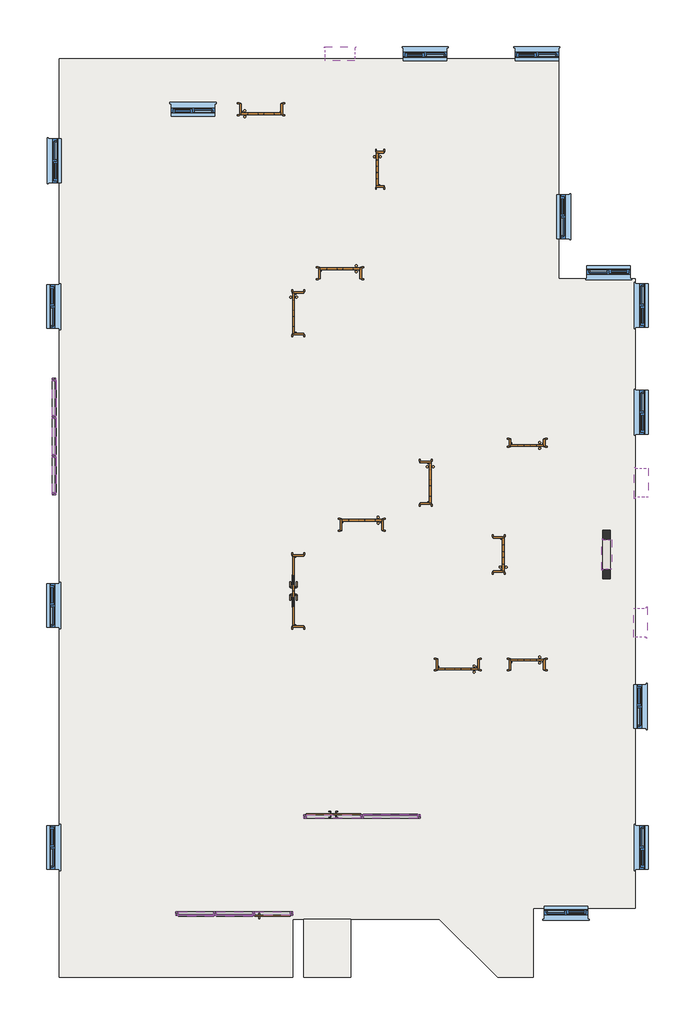
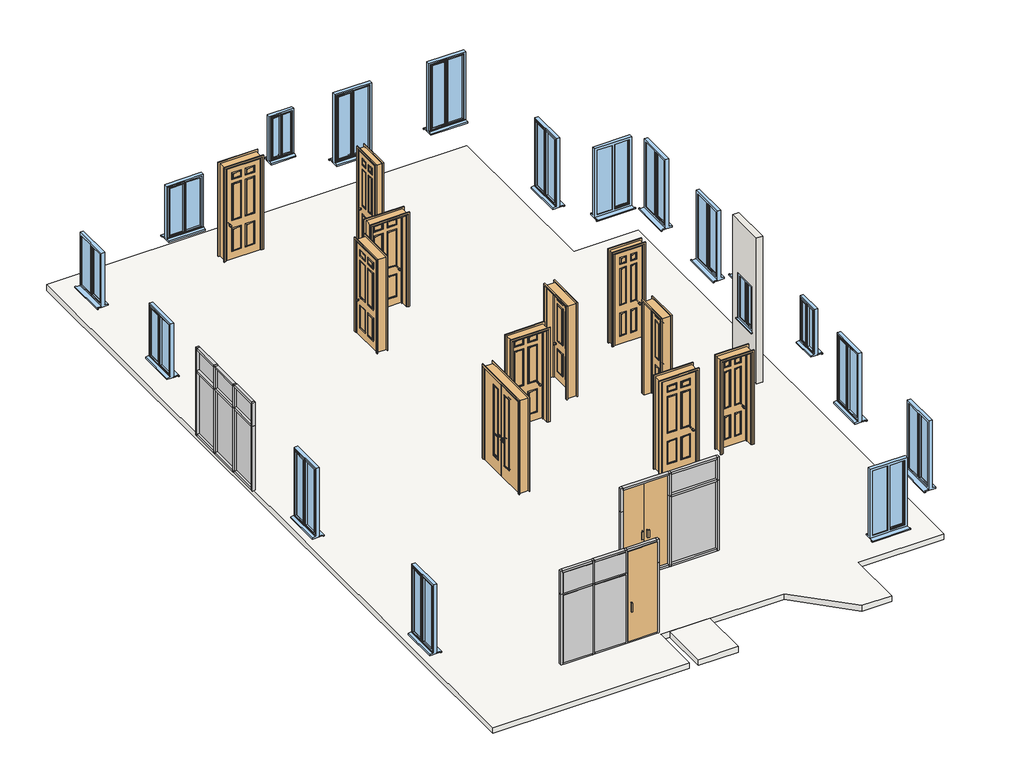
# One storey: 44 members, 18 windows, 13 doors, 12 plates, 2 slabs, 1 wall.
"""IFC4 building model written with IfcOpenShell, lengths in millimetres."""

from ifc_helpers import new_model, si_unit, frame, origin, place, context, project, spatial, polyline, outline, extrude, transform, mapped, element, save
from components import doors_intdbl_2_d4_7d0a9876, doors_intsgl_6_01_d1_adb953bf, doors_intsgl_6_01_d1_21fcec07, doors_intsgl_6_d2_0bf64c77, doors_intsgl_6_d2_b603f254, doors_intsgl_6_d2_ad12cddb, m_door_curtain_wall_double_glass_m_door_curtain_wall_double_ad7744c8, m_door_curtain_wall_single_glass_m_door_curtain_wall_single_7bb093da, rectangular_mullion_main_mullions_fa6a4a93, rectangular_mullion_main_mullions_32a4afb2, rectangular_mullion_main_mullions_07477f58, rectangular_mullion_main_mullions_65d9d1a0, rectangular_mullion_main_mullions_4e228a20, rectangular_mullion_main_mullions_6707c5fc, rectangular_mullion_main_mullions_bcbd968b, rectangular_mullion_main_mullions_6d09e4bf, rectangular_mullion_main_mullions_5bed117f, rectangular_mullion_main_mullions_97ba9194, rectangular_mullion_main_mullions_1ff2eda8, rectangular_mullion_main_mullions_8c683149, system_panel_glazed_41825f56, system_panel_glazed_b6ba8a14, system_panel_glazed_f19c5426, system_panel_glazed_62604723, system_panel_glazed_3b80f955, system_panel_glazed_1e8a61fc, system_panel_glazed_efe6ecb3, system_panel_glazed_1d3ea9f9, w1_9a3d44e1, w2_02e3e303, w2_3d16f0f7, w3_c0944c91

model = new_model("IFC4")

# Units and contexts
model_context = context("Model", 3, world=origin())
ifc_project = project(units=[si_unit("LENGTHUNIT", "METRE", prefix="MILLI")], contexts=[model_context])

# Site, building, storey
site = spatial("IfcSite", under=ifc_project)
building = spatial("IfcBuilding", under=site)
storey = spatial("IfcBuildingStorey", under=building, Elevation=600.0)

# Doors
placement = place(None, origin())
doors_intdbl_2_d4_shape = doors_intdbl_2_d4_7d0a9876(model_context)
element("IfcDoor", 1, ObjectType="Doors_IntDbl_2 : D4", at=placement, inside=storey, context=model_context, shape_type="MappedRepresentation", body=[
    mapped(doors_intdbl_2_d4_shape, transform((-3747.9564803, -5872.5265, 600.0), x_axis=(0.0, 1.0, 0.0), y_axis=(-1.0, 0.0, 0.0), z_axis=(0.0, 0.0, 1.0))),
])
doors_intsgl_6_01_d1_shape = doors_intsgl_6_01_d1_adb953bf(model_context)
element("IfcDoor", 2, ObjectType="Doors_IntSgl_6 : 01-D1", at=placement, inside=storey, context=model_context, shape_type="MappedRepresentation", body=[
    mapped(doors_intsgl_6_01_d1_shape, transform((-460.4564803, -7385.0265, 600.0), x_axis=(-1.0, 0.0, 0.0), y_axis=(0.0, -1.0, 0.0), z_axis=(0.0, 0.0, 1.0))),
])
element("IfcDoor", 3, ObjectType="Doors_IntSgl_6 : 01-D1", at=placement, inside=storey, context=model_context, shape_type="MappedRepresentation", body=[
    mapped(doors_intsgl_6_01_d1_shape, transform((-1122.9564803, -3647.5265, 600.0), x_axis=(0.0, -1.0, 0.0), y_axis=(1.0, 0.0, 0.0), z_axis=(0.0, 0.0, 1.0))),
])
doors_intsgl_6_01_d1_2_shape = doors_intsgl_6_01_d1_21fcec07(model_context)
element("IfcDoor", 4, ObjectType="Doors_IntSgl_6 : 01-D1", at=placement, inside=storey, context=model_context, shape_type="MappedRepresentation", body=[
    mapped(doors_intsgl_6_01_d1_2_shape, transform((-3747.9564803, -160.0265, 600.0), x_axis=(0.0, -1.0, 0.0), y_axis=(1.0, 0.0, 0.0), z_axis=(0.0, 0.0, 1.0))),
])
element("IfcDoor", 5, ObjectType="Doors_IntSgl_6 : 01-D1", at=placement, inside=storey, context=model_context, shape_type="MappedRepresentation", body=[
    mapped(doors_intsgl_6_01_d1_2_shape, transform((-4510.4564803, 4039.9735, 600.0), x_axis=(1.0, 0.0, 0.0), y_axis=(0.0, 1.0, 0.0), z_axis=(0.0, 0.0, 1.0))),
])
element("IfcDoor", 6, ObjectType="Doors_IntSgl_6 : 01-D1", at=placement, inside=storey, context=model_context, shape_type="MappedRepresentation", body=[
    mapped(doors_intsgl_6_01_d1_2_shape, transform((-2885.4564803, 664.9735, 600.0), x_axis=(-1.0, 0.0, 0.0), y_axis=(0.0, -1.0, 0.0), z_axis=(0.0, 0.0, 1.0))),
])
element("IfcDoor", 7, ObjectType="Doors_IntSgl_6 : 01-D1", at=placement, inside=storey, context=model_context, shape_type="MappedRepresentation", body=[
    mapped(doors_intsgl_6_01_d1_2_shape, transform((-2435.4564803, -4510.0265, 600.0), x_axis=(-1.0, 0.0, 0.0), y_axis=(0.0, -1.0, 0.0), z_axis=(0.0, 0.0, 1.0))),
])
doors_intsgl_6_d2_shape = doors_intsgl_6_d2_0bf64c77(model_context)
element("IfcDoor", 8, ObjectType="Doors_IntSgl_6 : D2", at=placement, inside=storey, context=model_context, shape_type="MappedRepresentation", body=[
    mapped(doors_intsgl_6_d2_shape, transform((377.0435197, -5122.5265, 600.0), x_axis=(0.0, 1.0, 0.0), y_axis=(-1.0, 0.0, 0.0), z_axis=(0.0, 0.0, 1.0))),
])
element("IfcDoor", 9, ObjectType="Doors_IntSgl_6 : D2", at=placement, inside=storey, context=model_context, shape_type="MappedRepresentation", body=[
    mapped(doors_intsgl_6_d2_shape, transform((964.5435197, -7385.0265, 600.0), x_axis=(-1.0, 0.0, 0.0), y_axis=(0.0, -1.0, 0.0), z_axis=(0.0, 0.0, 1.0))),
])
doors_intsgl_6_d2_2_shape = doors_intsgl_6_d2_b603f254(model_context)
element("IfcDoor", 10, ObjectType="Doors_IntSgl_6 : D2", at=placement, inside=storey, context=model_context, shape_type="MappedRepresentation", body=[
    mapped(doors_intsgl_6_d2_2_shape, transform((964.5435197, -2822.5265, 600.0), x_axis=(-1.0, 0.0, 0.0), y_axis=(0.0, -1.0, 0.0), z_axis=(0.0, 0.0, 1.0))),
])
doors_intsgl_6_d2_3_shape = doors_intsgl_6_d2_ad12cddb(model_context)
element("IfcDoor", 11, ObjectType="Doors_IntSgl_6 : D2", at=placement, inside=storey, context=model_context, shape_type="MappedRepresentation", body=[
    mapped(doors_intsgl_6_d2_3_shape, transform((-2060.4564803, 2802.4735, 600.0), x_axis=(0.0, -1.0, 0.0), y_axis=(1.0, 0.0, 0.0), z_axis=(0.0, 0.0, 1.0))),
])
m_door_curtain_wall_double_glass_m_door_curtain_wall_double_shape = m_door_curtain_wall_double_glass_m_door_curtain_wall_double_ad7744c8(model_context)
element("IfcDoor", 12, ObjectType="M_Door-Curtain-Wall-Double-Glass : M_Door-Curtain-Wall-Double-Glass", at=placement, inside=storey, context=model_context, shape_type="MappedRepresentation", body=[
    mapped(m_door_curtain_wall_double_glass_m_door_curtain_wall_double_shape, transform((-3022.9564803, -10510.0265, 650.0), x_axis=(1.0, 0.0, 0.0), y_axis=(0.0, 1.0, 0.0), z_axis=(0.0, 0.0, 1.0))),
])
m_door_curtain_wall_single_glass_m_door_curtain_wall_single_shape = m_door_curtain_wall_single_glass_m_door_curtain_wall_single_7bb093da(model_context)
element("IfcDoor", 13, ObjectType="M_Door-Curtain-Wall-Single-Glass : M_Door-Curtain-Wall-Single-Glass", at=placement, inside=storey, context=model_context, shape_type="MappedRepresentation", body=[
    mapped(m_door_curtain_wall_single_glass_m_door_curtain_wall_single_shape, transform((-4272.9564803, -12510.0265, 650.0), x_axis=(1.0, 0.0, 0.0), y_axis=(0.0, 1.0, 0.0), z_axis=(0.0, 0.0, 1.0))),
])

# Members
rectangular_mullion_main_mullions_shape = rectangular_mullion_main_mullions_fa6a4a93(model_context)
element("IfcMember", 14, ObjectType="Rectangular Mullion : main mullions", at=placement, inside=storey, context=model_context, shape_type="MappedRepresentation", body=[
    mapped(rectangular_mullion_main_mullions_shape, transform((-3860.4564803, -12510.0265, 3025.0), x_axis=(1.0, 0.0, 0.0), y_axis=(0.0, 1.0, 0.0), z_axis=(0.0, 0.0, 1.0))),
])
element("IfcMember", 15, ObjectType="Rectangular Mullion : main mullions", at=placement, inside=storey, context=model_context, shape_type="MappedRepresentation", body=[
    mapped(rectangular_mullion_main_mullions_shape, transform((-3635.4564803, -10510.0265, 3025.0), x_axis=(-1.0, 0.0, 0.0), y_axis=(0.0, -1.0, 0.0), z_axis=(0.0, 0.0, 1.0))),
])
rectangular_mullion_main_mullions_2_shape = rectangular_mullion_main_mullions_32a4afb2(model_context)
element("IfcMember", 16, ObjectType="Rectangular Mullion : main mullions", at=placement, inside=storey, context=model_context, shape_type="MappedRepresentation", body=[
    mapped(rectangular_mullion_main_mullions_2_shape, transform((-3860.4564803, -12510.0265, 2425.0), x_axis=(1.0, 0.0, 0.0), y_axis=(0.0, 1.0, 0.0), z_axis=(0.0, 0.0, 1.0))),
])
element("IfcMember", 17, ObjectType="Rectangular Mullion : main mullions", at=placement, inside=storey, context=model_context, shape_type="MappedRepresentation", body=[
    mapped(rectangular_mullion_main_mullions_2_shape, transform((-3635.4564803, -10510.0265, 2425.0), x_axis=(-1.0, 0.0, 0.0), y_axis=(0.0, -1.0, 0.0), z_axis=(0.0, 0.0, 1.0))),
])
rectangular_mullion_main_mullions_3_shape = rectangular_mullion_main_mullions_07477f58(model_context)
element("IfcMember", 18, ObjectType="Rectangular Mullion : main mullions", at=placement, inside=storey, context=model_context, shape_type="MappedRepresentation", body=[
    mapped(rectangular_mullion_main_mullions_3_shape, transform((-8772.9564803, -3847.5265, 3025.0), x_axis=(0.0, 0.0, 1.0), y_axis=(-1.0, 0.0, 0.0), z_axis=(0.0, -1.0, 0.0))),
])
element("IfcMember", 19, ObjectType="Rectangular Mullion : main mullions", at=placement, inside=storey, context=model_context, shape_type="MappedRepresentation", body=[
    mapped(rectangular_mullion_main_mullions_3_shape, transform((-6210.4564803, -12510.0265, 3025.0), x_axis=(0.0, 0.0, 1.0), y_axis=(0.0, 1.0, 0.0), z_axis=(-1.0, 0.0, 0.0))),
])
element("IfcMember", 20, ObjectType="Rectangular Mullion : main mullions", at=placement, inside=storey, context=model_context, shape_type="MappedRepresentation", body=[
    mapped(rectangular_mullion_main_mullions_3_shape, transform((-4635.4564803, -12510.0265, 3025.0), x_axis=(0.0, 0.0, 1.0), y_axis=(0.0, 1.0, 0.0), z_axis=(-1.0, 0.0, 0.0))),
])
element("IfcMember", 21, ObjectType="Rectangular Mullion : main mullions", at=placement, inside=storey, context=model_context, shape_type="MappedRepresentation", body=[
    mapped(rectangular_mullion_main_mullions_3_shape, transform((-8772.9564803, -2272.5265, 3025.0), x_axis=(0.0, 0.0, 1.0), y_axis=(-1.0, 0.0, 0.0), z_axis=(0.0, -1.0, 0.0))),
])
element("IfcMember", 22, ObjectType="Rectangular Mullion : main mullions", at=placement, inside=storey, context=model_context, shape_type="MappedRepresentation", body=[
    mapped(rectangular_mullion_main_mullions_3_shape, transform((-8772.9564803, -1547.5265, 750.0), x_axis=(0.0, 0.0, -1.0), y_axis=(-1.0, 0.0, 0.0), z_axis=(0.0, 1.0, 0.0))),
])
element("IfcMember", 23, ObjectType="Rectangular Mullion : main mullions", at=placement, inside=storey, context=model_context, shape_type="MappedRepresentation", body=[
    mapped(rectangular_mullion_main_mullions_3_shape, transform((-3910.4564803, -12510.0265, 600.0), x_axis=(0.0, 0.0, -1.0), y_axis=(0.0, 1.0, 0.0), z_axis=(1.0, 0.0, 0.0))),
])
element("IfcMember", 24, ObjectType="Rectangular Mullion : main mullions", at=placement, inside=storey, context=model_context, shape_type="MappedRepresentation", body=[
    mapped(rectangular_mullion_main_mullions_3_shape, transform((-5485.4564803, -12510.0265, 600.0), x_axis=(0.0, 0.0, -1.0), y_axis=(0.0, 1.0, 0.0), z_axis=(1.0, 0.0, 0.0))),
])
element("IfcMember", 25, ObjectType="Rectangular Mullion : main mullions", at=placement, inside=storey, context=model_context, shape_type="MappedRepresentation", body=[
    mapped(rectangular_mullion_main_mullions_3_shape, transform((-8772.9564803, -3122.5265, 750.0), x_axis=(0.0, 0.0, -1.0), y_axis=(-1.0, 0.0, 0.0), z_axis=(0.0, 1.0, 0.0))),
])
rectangular_mullion_main_mullions_4_shape = rectangular_mullion_main_mullions_65d9d1a0(model_context)
element("IfcMember", 26, ObjectType="Rectangular Mullion : main mullions", at=placement, inside=storey, context=model_context, shape_type="MappedRepresentation", body=[
    mapped(rectangular_mullion_main_mullions_4_shape, transform((-4685.4564803, -12510.0265, 600.0), x_axis=(0.0, 0.0, -1.0), y_axis=(0.0, 1.0, 0.0), z_axis=(1.0, 0.0, 0.0))),
])
element("IfcMember", 27, ObjectType="Rectangular Mullion : main mullions", at=placement, inside=storey, context=model_context, shape_type="MappedRepresentation", body=[
    mapped(rectangular_mullion_main_mullions_4_shape, transform((-8772.9564803, -2322.5265, 750.0), x_axis=(0.0, 0.0, -1.0), y_axis=(-1.0, 0.0, 0.0), z_axis=(0.0, 1.0, 0.0))),
])
element("IfcMember", 28, ObjectType="Rectangular Mullion : main mullions", at=placement, inside=storey, context=model_context, shape_type="MappedRepresentation", body=[
    mapped(rectangular_mullion_main_mullions_4_shape, transform((-5435.4564803, -12510.0265, 3025.0), x_axis=(0.0, 0.0, 1.0), y_axis=(0.0, 1.0, 0.0), z_axis=(-1.0, 0.0, 0.0))),
])
element("IfcMember", 29, ObjectType="Rectangular Mullion : main mullions", at=placement, inside=storey, context=model_context, shape_type="MappedRepresentation", body=[
    mapped(rectangular_mullion_main_mullions_4_shape, transform((-8772.9564803, -3072.5265, 3025.0), x_axis=(0.0, 0.0, 1.0), y_axis=(-1.0, 0.0, 0.0), z_axis=(0.0, -1.0, 0.0))),
])
rectangular_mullion_main_mullions_5_shape = rectangular_mullion_main_mullions_4e228a20(model_context)
element("IfcMember", 30, ObjectType="Rectangular Mullion : main mullions", at=placement, inside=storey, context=model_context, shape_type="MappedRepresentation", body=[
    mapped(rectangular_mullion_main_mullions_5_shape, transform((-8772.9564803, -2297.5265, 750.0), x_axis=(0.0, -1.0, 0.0), y_axis=(-1.0, 0.0, 0.0), z_axis=(0.0, 0.0, -1.0))),
])
element("IfcMember", 31, ObjectType="Rectangular Mullion : main mullions", at=placement, inside=storey, context=model_context, shape_type="MappedRepresentation", body=[
    mapped(rectangular_mullion_main_mullions_5_shape, transform((-8772.9564803, -3097.5265, 750.0), x_axis=(0.0, -1.0, 0.0), y_axis=(-1.0, 0.0, 0.0), z_axis=(0.0, 0.0, -1.0))),
])
rectangular_mullion_main_mullions_6_shape = rectangular_mullion_main_mullions_6707c5fc(model_context)
element("IfcMember", 32, ObjectType="Rectangular Mullion : main mullions", at=placement, inside=storey, context=model_context, shape_type="MappedRepresentation", body=[
    mapped(rectangular_mullion_main_mullions_6_shape, transform((-8772.9564803, -2272.5265, 2425.0), x_axis=(0.0, 0.0, 1.0), y_axis=(-1.0, 0.0, 0.0), z_axis=(0.0, -1.0, 0.0))),
])
element("IfcMember", 33, ObjectType="Rectangular Mullion : main mullions", at=placement, inside=storey, context=model_context, shape_type="MappedRepresentation", body=[
    mapped(rectangular_mullion_main_mullions_6_shape, transform((-8772.9564803, -3847.5265, 2425.0), x_axis=(0.0, 0.0, 1.0), y_axis=(-1.0, 0.0, 0.0), z_axis=(0.0, -1.0, 0.0))),
])
element("IfcMember", 34, ObjectType="Rectangular Mullion : main mullions", at=placement, inside=storey, context=model_context, shape_type="MappedRepresentation", body=[
    mapped(rectangular_mullion_main_mullions_6_shape, transform((-6210.4564803, -12510.0265, 2425.0), x_axis=(0.0, 0.0, 1.0), y_axis=(0.0, 1.0, 0.0), z_axis=(-1.0, 0.0, 0.0))),
])
rectangular_mullion_main_mullions_7_shape = rectangular_mullion_main_mullions_bcbd968b(model_context)
element("IfcMember", 35, ObjectType="Rectangular Mullion : main mullions", at=placement, inside=storey, context=model_context, shape_type="MappedRepresentation", body=[
    mapped(rectangular_mullion_main_mullions_7_shape, transform((-8772.9564803, -3072.5265, 2425.0), x_axis=(0.0, 0.0, 1.0), y_axis=(-1.0, 0.0, 0.0), z_axis=(0.0, -1.0, 0.0))),
])
element("IfcMember", 36, ObjectType="Rectangular Mullion : main mullions", at=placement, inside=storey, context=model_context, shape_type="MappedRepresentation", body=[
    mapped(rectangular_mullion_main_mullions_7_shape, transform((-5435.4564803, -12510.0265, 2425.0), x_axis=(0.0, 0.0, 1.0), y_axis=(0.0, 1.0, 0.0), z_axis=(-1.0, 0.0, 0.0))),
])
rectangular_mullion_main_mullions_8_shape = rectangular_mullion_main_mullions_6d09e4bf(model_context)
element("IfcMember", 37, ObjectType="Rectangular Mullion : main mullions", at=placement, inside=storey, context=model_context, shape_type="MappedRepresentation", body=[
    mapped(rectangular_mullion_main_mullions_8_shape, transform((-8772.9564803, -2297.5265, 2425.0), x_axis=(0.0, -1.0, 0.0), y_axis=(-1.0, 0.0, 0.0), z_axis=(0.0, 0.0, -1.0))),
])
element("IfcMember", 38, ObjectType="Rectangular Mullion : main mullions", at=placement, inside=storey, context=model_context, shape_type="MappedRepresentation", body=[
    mapped(rectangular_mullion_main_mullions_8_shape, transform((-8772.9564803, -3097.5265, 2425.0), x_axis=(0.0, -1.0, 0.0), y_axis=(-1.0, 0.0, 0.0), z_axis=(0.0, 0.0, -1.0))),
])
element("IfcMember", 39, ObjectType="Rectangular Mullion : main mullions", at=placement, inside=storey, context=model_context, shape_type="MappedRepresentation", body=[
    mapped(rectangular_mullion_main_mullions_8_shape, transform((-5460.4564803, -12510.0265, 2425.0), x_axis=(-1.0, 0.0, 0.0), y_axis=(0.0, 1.0, 0.0), z_axis=(0.0, 0.0, -1.0))),
])
element("IfcMember", 40, ObjectType="Rectangular Mullion : main mullions", at=placement, inside=storey, context=model_context, shape_type="MappedRepresentation", body=[
    mapped(rectangular_mullion_main_mullions_8_shape, transform((-4660.4564803, -12510.0265, 2425.0), x_axis=(-1.0, 0.0, 0.0), y_axis=(0.0, 1.0, 0.0), z_axis=(0.0, 0.0, -1.0))),
])
element("IfcMember", 41, ObjectType="Rectangular Mullion : main mullions", at=placement, inside=storey, context=model_context, shape_type="MappedRepresentation", body=[
    mapped(rectangular_mullion_main_mullions_8_shape, transform((-2435.4564803, -10510.0265, 2425.0), x_axis=(1.0, 0.0, 0.0), y_axis=(0.0, -1.0, 0.0), z_axis=(0.0, 0.0, -1.0))),
])
rectangular_mullion_main_mullions_9_shape = rectangular_mullion_main_mullions_5bed117f(model_context)
element("IfcMember", 42, ObjectType="Rectangular Mullion : main mullions", at=placement, inside=storey, context=model_context, shape_type="MappedRepresentation", body=[
    mapped(rectangular_mullion_main_mullions_9_shape, transform((-8772.9564803, -3897.5265, 750.0), x_axis=(0.0, -1.0, 0.0), y_axis=(-1.0, 0.0, 0.0), z_axis=(0.0, 0.0, -1.0))),
])
element("IfcMember", 43, ObjectType="Rectangular Mullion : main mullions", at=placement, inside=storey, context=model_context, shape_type="MappedRepresentation", body=[
    mapped(rectangular_mullion_main_mullions_shape, transform((-8772.9564803, -1497.5265, 3025.0), x_axis=(0.0, 1.0, 0.0), y_axis=(-1.0, 0.0, 0.0), z_axis=(0.0, 0.0, 1.0))),
])
element("IfcMember", 44, ObjectType="Rectangular Mullion : main mullions", at=placement, inside=storey, context=model_context, shape_type="MappedRepresentation", body=[
    mapped(rectangular_mullion_main_mullions_shape, transform((-6260.4564803, -12510.0265, 2425.0), x_axis=(-1.0, 0.0, 0.0), y_axis=(0.0, 1.0, 0.0), z_axis=(0.0, 0.0, -1.0))),
])
element("IfcMember", 45, ObjectType="Rectangular Mullion : main mullions", at=placement, inside=storey, context=model_context, shape_type="MappedRepresentation", body=[
    mapped(rectangular_mullion_main_mullions_shape, transform((-1235.4564803, -10510.0265, 2425.0), x_axis=(1.0, 0.0, 0.0), y_axis=(0.0, -1.0, 0.0), z_axis=(0.0, 0.0, -1.0))),
])
element("IfcMember", 46, ObjectType="Rectangular Mullion : main mullions", at=placement, inside=storey, context=model_context, shape_type="MappedRepresentation", body=[
    mapped(rectangular_mullion_main_mullions_shape, transform((-8772.9564803, -3897.5265, 2425.0), x_axis=(0.0, -1.0, 0.0), y_axis=(-1.0, 0.0, 0.0), z_axis=(0.0, 0.0, -1.0))),
])
element("IfcMember", 47, ObjectType="Rectangular Mullion : main mullions", at=placement, inside=storey, context=model_context, shape_type="MappedRepresentation", body=[
    mapped(rectangular_mullion_main_mullions_9_shape, transform((-8772.9564803, -1497.5265, 2425.0), x_axis=(0.0, 1.0, 0.0), y_axis=(-1.0, 0.0, 0.0), z_axis=(0.0, 0.0, 1.0))),
])
rectangular_mullion_main_mullions_10_shape = rectangular_mullion_main_mullions_97ba9194(model_context)
element("IfcMember", 48, ObjectType="Rectangular Mullion : main mullions", at=placement, inside=storey, context=model_context, shape_type="MappedRepresentation", body=[
    mapped(rectangular_mullion_main_mullions_10_shape, transform((-5460.4564803, -12510.0265, 600.0), x_axis=(-1.0, 0.0, 0.0), y_axis=(0.0, 1.0, 0.0), z_axis=(0.0, 0.0, -1.0))),
])
element("IfcMember", 49, ObjectType="Rectangular Mullion : main mullions", at=placement, inside=storey, context=model_context, shape_type="MappedRepresentation", body=[
    mapped(rectangular_mullion_main_mullions_10_shape, transform((-4660.4564803, -12510.0265, 600.0), x_axis=(-1.0, 0.0, 0.0), y_axis=(0.0, 1.0, 0.0), z_axis=(0.0, 0.0, -1.0))),
])
element("IfcMember", 50, ObjectType="Rectangular Mullion : main mullions", at=placement, inside=storey, context=model_context, shape_type="MappedRepresentation", body=[
    mapped(rectangular_mullion_main_mullions_10_shape, transform((-2435.4564803, -10510.0265, 600.0), x_axis=(1.0, 0.0, 0.0), y_axis=(0.0, -1.0, 0.0), z_axis=(0.0, 0.0, -1.0))),
])
element("IfcMember", 51, ObjectType="Rectangular Mullion : main mullions", at=placement, inside=storey, context=model_context, shape_type="MappedRepresentation", body=[
    mapped(rectangular_mullion_main_mullions_2_shape, transform((-6260.4564803, -12510.0265, 600.0), x_axis=(-1.0, 0.0, 0.0), y_axis=(0.0, 1.0, 0.0), z_axis=(0.0, 0.0, -1.0))),
])
element("IfcMember", 52, ObjectType="Rectangular Mullion : main mullions", at=placement, inside=storey, context=model_context, shape_type="MappedRepresentation", body=[
    mapped(rectangular_mullion_main_mullions_2_shape, transform((-1235.4564803, -10510.0265, 600.0), x_axis=(1.0, 0.0, 0.0), y_axis=(0.0, -1.0, 0.0), z_axis=(0.0, 0.0, -1.0))),
])
rectangular_mullion_main_mullions_11_shape = rectangular_mullion_main_mullions_1ff2eda8(model_context)
element("IfcMember", 53, ObjectType="Rectangular Mullion : main mullions", at=placement, inside=storey, context=model_context, shape_type="MappedRepresentation", body=[
    mapped(rectangular_mullion_main_mullions_11_shape, transform((-1285.4564803, -10510.0265, 3025.0), x_axis=(0.0, 0.0, 1.0), y_axis=(0.0, -1.0, 0.0), z_axis=(1.0, 0.0, 0.0))),
])
element("IfcMember", 54, ObjectType="Rectangular Mullion : main mullions", at=placement, inside=storey, context=model_context, shape_type="MappedRepresentation", body=[
    mapped(rectangular_mullion_main_mullions_11_shape, transform((-2460.4564803, -10510.0265, 3025.0), x_axis=(0.0, 0.0, 1.0), y_axis=(0.0, -1.0, 0.0), z_axis=(1.0, 0.0, 0.0))),
])
element("IfcMember", 55, ObjectType="Rectangular Mullion : main mullions", at=placement, inside=storey, context=model_context, shape_type="MappedRepresentation", body=[
    mapped(rectangular_mullion_main_mullions_11_shape, transform((-3585.4564803, -10510.0265, 600.0), x_axis=(0.0, 0.0, -1.0), y_axis=(0.0, -1.0, 0.0), z_axis=(-1.0, 0.0, 0.0))),
])
element("IfcMember", 56, ObjectType="Rectangular Mullion : main mullions", at=placement, inside=storey, context=model_context, shape_type="MappedRepresentation", body=[
    mapped(rectangular_mullion_main_mullions_11_shape, transform((-2410.4564803, -10510.0265, 600.0), x_axis=(0.0, 0.0, -1.0), y_axis=(0.0, -1.0, 0.0), z_axis=(-1.0, 0.0, 0.0))),
])
rectangular_mullion_main_mullions_12_shape = rectangular_mullion_main_mullions_8c683149(model_context)
element("IfcMember", 57, ObjectType="Rectangular Mullion : main mullions", at=placement, inside=storey, context=model_context, shape_type="MappedRepresentation", body=[
    mapped(rectangular_mullion_main_mullions_12_shape, transform((-1285.4564803, -10510.0265, 2425.0), x_axis=(0.0, 0.0, 1.0), y_axis=(0.0, -1.0, 0.0), z_axis=(1.0, 0.0, 0.0))),
])

# Plates
system_panel_glazed_shape = system_panel_glazed_41825f56(model_context)
element("IfcPlate", 58, ObjectType="System Panel : Glazed", at=placement, inside=storey, context=model_context, shape_type="MappedRepresentation", body=[
    mapped(system_panel_glazed_shape, transform((-8772.9564803, -1910.0265, 800.0), x_axis=(0.0, -1.0, 0.0), y_axis=(1.0, 0.0, 0.0), z_axis=(0.0, 0.0, 1.0))),
])
element("IfcPlate", 59, ObjectType="System Panel : Glazed", at=placement, inside=storey, context=model_context, shape_type="MappedRepresentation", body=[
    mapped(system_panel_glazed_shape, transform((-8772.9564803, -3485.0265, 800.0), x_axis=(0.0, -1.0, 0.0), y_axis=(1.0, 0.0, 0.0), z_axis=(0.0, 0.0, 1.0))),
])
system_panel_glazed_2_shape = system_panel_glazed_b6ba8a14(model_context)
element("IfcPlate", 60, ObjectType="System Panel : Glazed", at=placement, inside=storey, context=model_context, shape_type="MappedRepresentation", body=[
    mapped(system_panel_glazed_2_shape, transform((-8772.9564803, -2697.5265, 800.0), x_axis=(0.0, -1.0, 0.0), y_axis=(1.0, 0.0, 0.0), z_axis=(0.0, 0.0, 1.0))),
])
system_panel_glazed_3_shape = system_panel_glazed_f19c5426(model_context)
element("IfcPlate", 61, ObjectType="System Panel : Glazed", at=placement, inside=storey, context=model_context, shape_type="MappedRepresentation", body=[
    mapped(system_panel_glazed_3_shape, transform((-5847.9564803, -12510.0265, 2450.0), x_axis=(-1.0, 0.0, 0.0), y_axis=(0.0, -1.0, 0.0), z_axis=(0.0, 0.0, 1.0))),
])
element("IfcPlate", 62, ObjectType="System Panel : Glazed", at=placement, inside=storey, context=model_context, shape_type="MappedRepresentation", body=[
    mapped(system_panel_glazed_3_shape, transform((-8772.9564803, -1910.0265, 2450.0), x_axis=(0.0, -1.0, 0.0), y_axis=(1.0, 0.0, 0.0), z_axis=(0.0, 0.0, 1.0))),
])
element("IfcPlate", 63, ObjectType="System Panel : Glazed", at=placement, inside=storey, context=model_context, shape_type="MappedRepresentation", body=[
    mapped(system_panel_glazed_3_shape, transform((-8772.9564803, -3485.0265, 2450.0), x_axis=(0.0, -1.0, 0.0), y_axis=(1.0, 0.0, 0.0), z_axis=(0.0, 0.0, 1.0))),
])
system_panel_glazed_4_shape = system_panel_glazed_62604723(model_context)
element("IfcPlate", 64, ObjectType="System Panel : Glazed", at=placement, inside=storey, context=model_context, shape_type="MappedRepresentation", body=[
    mapped(system_panel_glazed_4_shape, transform((-5060.4564803, -12510.0265, 2450.0), x_axis=(-1.0, 0.0, 0.0), y_axis=(0.0, -1.0, 0.0), z_axis=(0.0, 0.0, 1.0))),
])
element("IfcPlate", 65, ObjectType="System Panel : Glazed", at=placement, inside=storey, context=model_context, shape_type="MappedRepresentation", body=[
    mapped(system_panel_glazed_4_shape, transform((-8772.9564803, -2697.5265, 2450.0), x_axis=(0.0, -1.0, 0.0), y_axis=(1.0, 0.0, 0.0), z_axis=(0.0, 0.0, 1.0))),
])
system_panel_glazed_5_shape = system_panel_glazed_3b80f955(model_context)
element("IfcPlate", 66, ObjectType="System Panel : Glazed", at=placement, inside=storey, context=model_context, shape_type="MappedRepresentation", body=[
    mapped(system_panel_glazed_5_shape, transform((-5847.9564803, -12510.0265, 650.0), x_axis=(-1.0, 0.0, 0.0), y_axis=(0.0, -1.0, 0.0), z_axis=(0.0, 0.0, 1.0))),
])
system_panel_glazed_6_shape = system_panel_glazed_1e8a61fc(model_context)
element("IfcPlate", 67, ObjectType="System Panel : Glazed", at=placement, inside=storey, context=model_context, shape_type="MappedRepresentation", body=[
    mapped(system_panel_glazed_6_shape, transform((-5060.4564803, -12510.0265, 650.0), x_axis=(-1.0, 0.0, 0.0), y_axis=(0.0, -1.0, 0.0), z_axis=(0.0, 0.0, 1.0))),
])
system_panel_glazed_7_shape = system_panel_glazed_efe6ecb3(model_context)
element("IfcPlate", 68, ObjectType="System Panel : Glazed", at=placement, inside=storey, context=model_context, shape_type="MappedRepresentation", body=[
    mapped(system_panel_glazed_7_shape, transform((-1847.9564803, -10510.0265, 650.0), x_axis=(1.0, 0.0, 0.0), y_axis=(0.0, 1.0, 0.0), z_axis=(0.0, 0.0, 1.0))),
])
system_panel_glazed_8_shape = system_panel_glazed_1d3ea9f9(model_context)
element("IfcPlate", 69, ObjectType="System Panel : Glazed", at=placement, inside=storey, context=model_context, shape_type="MappedRepresentation", body=[
    mapped(system_panel_glazed_8_shape, transform((-1847.9564803, -10510.0265, 2450.0), x_axis=(1.0, 0.0, 0.0), y_axis=(0.0, 1.0, 0.0), z_axis=(0.0, 0.0, 1.0))),
])

# Slabs
element("IfcSlab", 70, ObjectType="01- floor main", at=placement, inside=storey, context=model_context, shape_type="SweptSolid", body=[
    extrude(outline(polyline([(1614.5435197, 5077.4735), (1614.5435197, 552.4735), (3189.5435197, 552.4735), (3189.5435197, -12397.5265), (1089.5435197, -12397.5265), (1089.5435197, -13822.5265), (357.7415713, -13822.5265), (-842.2584287, -12622.5265), (-3860.4564803, -12622.5265), (-3860.4564803, -13822.5265), (-8660.4564803, -13822.5265), (-8660.4564803, 5077.4735), (1614.5435197, 5077.4735)])), frame((0.0, 0.0, 450.0), z_axis=(0.0, 0.0, 1.0), x_axis=(1.0, 0.0, 0.0)), (0.0, 0.0, 1.0), 150.0),
])
element("IfcSlab", 71, ObjectType="03-green area", at=placement, inside=storey, context=model_context, shape_type="SweptSolid", body=[
    extrude(outline(polyline([(-2660.4564803, -12622.5265), (-2660.4564803, -13822.5265), (-3635.4564803, -13822.5265), (-3635.4564803, -12622.5265), (-2660.4564803, -12622.5265)])), frame((0.0, 0.0, 450.0), z_axis=(0.0, 0.0, 1.0), x_axis=(1.0, 0.0, 0.0)), (0.0, 0.0, 1.0), 150.0),
])

# Wall
element("IfcWall", 72, ObjectType="02-150 WALL", at=placement, inside=storey, context=model_context, shape_type="SweptSolid", body=[
    extrude(outline(polyline([(-4622.5265, 600.0), (-5622.5265, 600.0), (-5622.5265, 4375.0), (-4622.5265, 4375.0), (-4622.5265, 600.0)]), holes=[polyline([(-4822.5265, 3000.0), (-5422.5265, 3000.0), (-5422.5265, 1800.0), (-4822.5265, 1800.0), (-4822.5265, 3000.0)])]), frame((2519.5435197, 0.0, 0.0), z_axis=(1.0, 0.0, 0.0), x_axis=(0.0, 1.0, 0.0)), (0.0, 0.0, 1.0), 150.0),
])

# Windows
w1_shape = w1_9a3d44e1(model_context)
element("IfcWindow", 73, ObjectType="W1", at=placement, inside=storey, context=model_context, shape_type="MappedRepresentation", body=[
    mapped(w1_shape, transform((-8764.4999124, -10862.5265, 600.0), x_axis=(0.0, 1.0, 0.0), y_axis=(-1.0, 0.0, 0.0), z_axis=(0.0, 0.0, 1.0))),
])
element("IfcWindow", 74, ObjectType="W1", at=placement, inside=storey, context=model_context, shape_type="MappedRepresentation", body=[
    mapped(w1_shape, transform((-8764.4999124, -5887.5265, 600.0), x_axis=(0.0, 1.0, 0.0), y_axis=(-1.0, 0.0, 0.0), z_axis=(0.0, 0.0, 1.0))),
])
element("IfcWindow", 75, ObjectType="W1", at=placement, inside=storey, context=model_context, shape_type="MappedRepresentation", body=[
    mapped(w1_shape, transform((2049.5435197, -12518.4830678, 600.0), x_axis=(1.0, 0.0, 0.0), y_axis=(0.0, 1.0, 0.0), z_axis=(0.0, 0.0, 1.0))),
])
element("IfcWindow", 76, ObjectType="W1", at=placement, inside=storey, context=model_context, shape_type="MappedRepresentation", body=[
    mapped(w1_shape, transform((3293.5869519, -11432.5265, 600.0), x_axis=(0.0, -1.0, 0.0), y_axis=(1.0, 0.0, 0.0), z_axis=(0.0, 0.0, 1.0))),
])
element("IfcWindow", 77, ObjectType="W1", at=placement, inside=storey, context=model_context, shape_type="MappedRepresentation", body=[
    mapped(w1_shape, transform((3310.5000876, -7962.5265, 600.0), x_axis=(0.0, 1.0, 0.0), y_axis=(-1.0, 0.0, 0.0), z_axis=(0.0, 0.0, 1.0))),
])
element("IfcWindow", 78, ObjectType="W1", at=placement, inside=storey, context=model_context, shape_type="MappedRepresentation", body=[
    mapped(w1_shape, transform((3293.5869519, -2482.5265, 600.0), x_axis=(0.0, -1.0, 0.0), y_axis=(1.0, 0.0, 0.0), z_axis=(0.0, 0.0, 1.0))),
])
element("IfcWindow", 79, ObjectType="W1", at=placement, inside=storey, context=model_context, shape_type="MappedRepresentation", body=[
    mapped(w1_shape, transform((3293.5869519, -282.5265, 600.0), x_axis=(0.0, -1.0, 0.0), y_axis=(1.0, 0.0, 0.0), z_axis=(0.0, 0.0, 1.0))),
])
element("IfcWindow", 80, ObjectType="W1", at=placement, inside=storey, context=model_context, shape_type="MappedRepresentation", body=[
    mapped(w1_shape, transform((2924.5435197, 656.5169322, 600.0), x_axis=(1.0, 0.0, 0.0), y_axis=(0.0, 1.0, 0.0), z_axis=(0.0, 0.0, 1.0))),
])
element("IfcWindow", 81, ObjectType="W1", at=placement, inside=storey, context=model_context, shape_type="MappedRepresentation", body=[
    mapped(w1_shape, transform((1735.5000876, 2112.4735, 600.0), x_axis=(0.0, 1.0, 0.0), y_axis=(-1.0, 0.0, 0.0), z_axis=(0.0, 0.0, 1.0))),
])
element("IfcWindow", 82, ObjectType="W1", at=placement, inside=storey, context=model_context, shape_type="MappedRepresentation", body=[
    mapped(w1_shape, transform((879.5435197, 5198.4300678, 600.0), x_axis=(-1.0, 0.0, 0.0), y_axis=(0.0, -1.0, 0.0), z_axis=(0.0, 0.0, 1.0))),
])
element("IfcWindow", 83, ObjectType="W1", at=placement, inside=storey, context=model_context, shape_type="MappedRepresentation", body=[
    mapped(w1_shape, transform((-1420.4564803, 5198.4300678, 600.0), x_axis=(-1.0, 0.0, 0.0), y_axis=(0.0, -1.0, 0.0), z_axis=(0.0, 0.0, 1.0))),
])
w2_shape = w2_02e3e303(model_context)
element("IfcWindow", 84, ObjectType="W2", at=placement, inside=storey, context=model_context, shape_type="MappedRepresentation", body=[
    mapped(w2_shape, transform((3310.5000876, -6237.5265, 600.0), x_axis=(0.0, 1.0, 0.0), y_axis=(-1.0, 0.0, 0.0), z_axis=(0.0, 0.0, 1.0))),
])
element("IfcWindow", 85, ObjectType="W2", at=placement, inside=storey, context=model_context, shape_type="MappedRepresentation", body=[
    mapped(w2_shape, transform((3293.5869519, -3932.5265, 600.0), x_axis=(0.0, -1.0, 0.0), y_axis=(1.0, 0.0, 0.0), z_axis=(0.0, 0.0, 1.0))),
])
element("IfcWindow", 86, ObjectType="W2", at=placement, inside=storey, context=model_context, shape_type="MappedRepresentation", body=[
    mapped(w2_shape, transform((-3170.4564803, 5198.4300678, 600.0), x_axis=(-1.0, 0.0, 0.0), y_axis=(0.0, -1.0, 0.0), z_axis=(0.0, 0.0, 1.0))),
])
w2_2_shape = w2_3d16f0f7(model_context)
element("IfcWindow", 87, ObjectType="W2", at=placement, inside=storey, context=model_context, shape_type="MappedRepresentation", body=[
    mapped(w2_2_shape, transform((2586.0869519, -5407.5265, 600.0), x_axis=(0.0, -1.0, 0.0), y_axis=(1.0, 0.0, 0.0), z_axis=(0.0, 0.0, 1.0))),
])
w3_shape = w3_c0944c91(model_context)
element("IfcWindow", 88, ObjectType="W3", at=placement, inside=storey, context=model_context, shape_type="MappedRepresentation", body=[
    mapped(w3_shape, transform((-6195.4564803, 4048.4300678, 600.0), x_axis=(-1.0, 0.0, 0.0), y_axis=(0.0, -1.0, 0.0), z_axis=(0.0, 0.0, 1.0))),
])
element("IfcWindow", 89, ObjectType="W3", at=placement, inside=storey, context=model_context, shape_type="MappedRepresentation", body=[
    mapped(w3_shape, transform((-8781.4130481, 2692.4735, 600.0), x_axis=(0.0, -1.0, 0.0), y_axis=(1.0, 0.0, 0.0), z_axis=(0.0, 0.0, 1.0))),
])
element("IfcWindow", 90, ObjectType="W3", at=placement, inside=storey, context=model_context, shape_type="MappedRepresentation", body=[
    mapped(w3_shape, transform((-8764.4999124, 262.4735, 600.0), x_axis=(0.0, 1.0, 0.0), y_axis=(-1.0, 0.0, 0.0), z_axis=(0.0, 0.0, 1.0))),
])

save(model, "model.ifc")

# Revit data of these elements
# Type "Doors_IntDbl_2 : D4"
#   Type Mark = "55"
#   Type Comments = "Internal Double"
#   Operation = "DoubleDoorSingleSwing"
#   Construction Type Id = "GSP4R"
#   Keynote = "L20"
#   Description = "Internal Double Door"
#   Analytic Construction = "1/8 in Pilkington single glazing"
#   Visual Light Transmittance = 0.9
#   VisionPanel Width = 200 mm
#   Thickness = 32 mm
#   Stop Thickness = 19 mm
#   Stop Depth = 32 mm
#   Stile Top Rail = 225 mm
#   Stile Shutting = 125 mm
#   Stile Bottom Rail = 350 mm
#   Solar Heat Gain Coefficient = 0.78
#   Rough Width = 1500 mm
#   Rough Height = 2400 mm
#   Heat Transfer Coefficient (U) = 3.6886 W/(m²·K)
#   Handle Z Distance = 1000 mm
#   Handle X Distance = 75 mm
#   Frame Thickness = 32 mm
#   Door Panel Width = 705.5 mm
#   Door Panel Thickness = 32 mm
#   Door Panel Height = 2350 mm
#   Height = 2400 mm
#   Door Panel Offset = 0 mm
#   Structural Tolerance = 8 mm
#   Tolerance = 3 mm
#   UnderCut = 7 mm
#   Width = 1500 mm
#   Architrave Setback = 5 mm
#   Vis - Ironmongery = yes
#   Define Thermal Properties by = 1
#   Material Ironmongery = Door - Handle
#   Material Glass = Door - Glazing
#   Material Frame = Door - Frame/Mullion
#   Material Door = Door - Panel
#   Material Beading = Door - Panel
#   Material Architrave = Door - Architrave
#   Function = (empty or 0)
#   Wall Closure = (empty or 0)
# Type "Doors_IntSgl_6 : 01-D1"
#   Type Mark = "49"
#   Type Comments = "Internal Single"
#   Operation = "SingleSwingRight"
#   Construction Type Id = "MDOOR"
#   Manufacturer = "Revit"
#   Keynote = "L20"
#   Description = "Internal Single Door"
#   Analytic Construction = "Metal"
#   UnderCut = 8 mm
#   Tolerance = 2 mm
#   Thickness = 38 mm
#   Structural Tolerance = 8 mm
#   StopDepth = 32 mm
#   Stop Thickness = 19 mm
#   Stile Top Rail = 125 mm
#   Stile Shutting = 125 mm
#   Stile Muntin Rail = 100 mm
#   Stile Lock Rail = 200 mm
#   Stile Intermediate/Frieze = 100 mm
#   Stile Hanging = 125 mm
#   Stile Bottom Rail = 200 mm
#   Rough Width = 900 mm
#   Rough Height = 2400 mm
#   Height to Top Lock Rail = 1000 mm
#   Heat Transfer Coefficient (U) = 3.7021 W/(m²·K)
#   Handle Z Distance = 900 mm
#   Handle X Distance = 75 mm
#   Frame Thickness = 32 mm
#   Door Panel Width = 816 mm
#   Height = 2400 mm
#   Width = 900 mm
#   Door Panel Thickness = 38 mm
#   Door Panel Offset = 0 mm
#   Door Panel Height = 2350 mm
#   Architrave Setback = 5 mm
#   Vis - Ironmongery = yes
#   Define Thermal Properties by = 1
#   Material Ironmongery = Door - Handle
#   Material Frame = Door - Frame/Mullion
#   Material Door = Door - Panel
#   Material Architrave = Door - Architrave
#   Visual Light Transmittance = 0
#   Solar Heat Gain Coefficient = 0
#   Function = (empty or 0)
#   Wall Closure = (empty or 0)
# Type "Doors_IntSgl_6 : D2"
#   Type Mark = "50"
#   Type Comments = "Internal Single"
#   Operation = "SingleSwingRight"
#   Construction Type Id = "MDOOR"
#   Manufacturer = "Revit"
#   Keynote = "L20"
#   Description = "Internal Single Door"
#   Analytic Construction = "Metal"
#   UnderCut = 8 mm
#   Tolerance = 2 mm
#   Thickness = 38 mm
#   Structural Tolerance = 8 mm
#   StopDepth = 32 mm
#   Stop Thickness = 19 mm
#   Stile Top Rail = 125 mm
#   Stile Shutting = 125 mm
#   Stile Muntin Rail = 100 mm
#   Stile Lock Rail = 200 mm
#   Stile Intermediate/Frieze = 100 mm
#   Stile Hanging = 125 mm
#   Stile Bottom Rail = 200 mm
#   Rough Width = 750 mm
#   Rough Height = 2400 mm
#   Height to Top Lock Rail = 1000 mm
#   Heat Transfer Coefficient (U) = 3.7021 W/(m²·K)
#   Handle Z Distance = 900 mm
#   Handle X Distance = 75 mm
#   Frame Thickness = 32 mm
#   Door Panel Width = 666 mm
#   Height = 2400 mm
#   Width = 750 mm
#   Door Panel Thickness = 38 mm
#   Door Panel Offset = 0 mm
#   Door Panel Height = 2350 mm
#   Architrave Setback = 5 mm
#   Vis - Ironmongery = yes
#   Define Thermal Properties by = 1
#   Material Ironmongery = Door - Handle
#   Material Frame = Door - Frame/Mullion
#   Material Door = Door - Panel
#   Material Architrave = Door - Architrave
#   Visual Light Transmittance = 0
#   Solar Heat Gain Coefficient = 0
#   Function = (empty or 0)
#   Wall Closure = (empty or 0)
# Type "M_Door-Curtain-Wall-Double-Glass : M_Door-Curtain-Wall-Double-Glass"
#   Type Mark = "47"
#   Assembly Code = "B2030100"
#   Analytic Construction = "<None>"
#   Width [instance default] = 1800 mm
#   Thermal Resistance (R) = 1.7611 (m²·K)/W
#   Swing Angle [instance default] = 90.00°
#   Panel Width [instance default] = 900 mm
#   Offset = 50.8 mm
#   Heat Transfer Coefficient (U) = 0.567826 W/(m²·K)
#   Define Thermal Properties by = 1
#   Function = 1
#   Door Handle Material = Aluminum
#   Glazing = Glass
#   Visual Light Transmittance = 0
#   Solar Heat Gain Coefficient = 0
#   Construction Type Id = ""
# Type "M_Door-Curtain-Wall-Single-Glass : M_Door-Curtain-Wall-Single-Glass"
#   Type Mark = "46"
#   Assembly Code = "B2030100"
#   Analytic Construction = "<None>"
#   Width [instance default] = 900 mm
#   Thermal Resistance (R) = 1.7611 (m²·K)/W
#   Swing Angle [instance default] = 90.00°
#   Heat Transfer Coefficient (U) = 0.567826 W/(m²·K)
#   Offset = 50.8 mm
#   Define Thermal Properties by = 1
#   Function = 1
#   Door Handle Material = Aluminum
#   Glazing = Glass
#   Visual Light Transmittance = 0
#   Solar Heat Gain Coefficient = 0
#   Construction Type Id = ""
# Type "Rectangular Mullion : main mullions"
#   built-in parameter 1007304 = 0.246063 (stored number, unit not read)
#   built-in parameter 1007301 = 0.082021 (stored number, unit not read)
#   built-in parameter 1007300 = 0.082021 (stored number, unit not read)
# Type "System Panel : Glazed"
#   Construction Type Id = "GSP4R"
#   Analytic Construction = "1/8 in Pilkington single glazing"
#   Visual Light Transmittance = 0.9
#   Solar Heat Gain Coefficient = 0.86
#   Heat Transfer Coefficient (U) = 6.7069 W/(m²·K)
#   Define Thermal Properties by = 1
# Type "01- floor main"
#   Description = "Generic Floor (Material By Category), 12\" thick"
#   Assembly Code = "B1010"
#   Type Mark = "G01"
#   Function = 0
#   Layers, outside or top first: 150 mm "02-floor tile" (function 1)
# Type "03-green area"
#   Description = "Generic Floor (Material By Category), 12\" thick"
#   Assembly Code = "B1010"
#   Type Mark = "G01"
#   Function = 0
#   Layers, outside or top first: 150 mm "03-green area" (function 1)
# Type "02-150 WALL"
#   Description = "Generic Wall (Material By Category), 200mm thick"
#   Assembly Code = "B2010"
#   Type Mark = "G06"
#   Layers, outside or top first: 150 mm "01-225 wall paint" (function 1)
# Type "W1"
#   Type Mark = "40"
#   Operation = "DoublePanelVertical"
#   Manufacturer = "Revit"
#   Wrap Layers (Ext) from Ext = 102.5 mm
#   Wrap Layers (Int) from Ext = 177.5 mm
#   Window Board Projection = 25 mm
#   Window Board Extension = 25 mm
#   Rough Width = 900 mm
#   Rough Height = 1800 mm
#   Height = 1800 mm
#   Width = 900 mm
#   Glazing Thickness = 24 mm
#   FrameOffset - External = 50 mm
#   Frame Depth = 65 mm
#   Default Head Height = 2400 mm
#   Cill Depth = 87.5 mm
#   Cavity Closer Width = 50 mm
#   Cavity Closer Offset from Ext = 102.5 mm
#   Cavity Closer Depth = 85 mm
#   Vis - Cavity Closers = yes
#   Material Trim = Window Frame
#   Material Glass = Glass
#   Material Frame = Window Frame
#   Wall Closure = (empty or 0)
# Type "W2"
#   Type Mark = "42"
#   Operation = "DoublePanelVertical"
#   Manufacturer = "Revit"
#   Wrap Layers (Ext) from Ext = 102.5 mm
#   Wrap Layers (Int) from Ext = 177.5 mm
#   Window Board Projection = 25 mm
#   Window Board Extension = 25 mm
#   Rough Width = 600 mm
#   Rough Height = 1200 mm
#   Height = 1200 mm
#   Width = 600 mm
#   Glazing Thickness = 24 mm
#   FrameOffset - External = 50 mm
#   Frame Depth = 65 mm
#   Default Head Height = 2400 mm
#   Cill Depth = 87.5 mm
#   Cavity Closer Width = 50 mm
#   Cavity Closer Offset from Ext = 102.5 mm
#   Cavity Closer Depth = 85 mm
#   Vis - Cavity Closers = yes
#   Material Trim = Window Frame
#   Material Glass = Glass
#   Material Frame = Window Frame
#   Wall Closure = (empty or 0)
# Type "W3"
#   Type Mark = "41"
#   Operation = "DoublePanelVertical"
#   Manufacturer = "Revit"
#   Wrap Layers (Ext) from Ext = 102.5 mm
#   Wrap Layers (Int) from Ext = 177.5 mm
#   Window Board Projection = 25 mm
#   Window Board Extension = 25 mm
#   Rough Width = 900 mm
#   Rough Height = 1400 mm
#   Height = 1400 mm
#   Width = 900 mm
#   Glazing Thickness = 24 mm
#   FrameOffset - External = 50 mm
#   Frame Depth = 65 mm
#   Default Head Height = 2400 mm
#   Cill Depth = 87.5 mm
#   Cavity Closer Width = 50 mm
#   Cavity Closer Offset from Ext = 102.5 mm
#   Cavity Closer Depth = 85 mm
#   Vis - Cavity Closers = yes
#   Material Trim = Window Frame
#   Material Glass = Glass
#   Material Frame = Window Frame
#   Wall Closure = (empty or 0)
# Element 1 (IfcDoor, "Doors_IntDbl_2 : D4")
#   Phase Created = New Construction
#   Materials on its faces: "Door - Panel", "Door - Handle", "Door - Architrave", "Door - Frame/Mullion", "Door - Glazing"
# Elements 2, 3, 4, 5, 6, 7 (IfcDoor, "Doors_IntSgl_6 : 01-D1")
#   Phase Created = New Construction
#   Materials on its faces: "Door - Panel", "Door - Architrave", "Door - Frame/Mullion", "Door - Handle"
# Elements 8, 9, 10, 11 (IfcDoor, "Doors_IntSgl_6 : D2")
#   Phase Created = New Construction
#   Materials on its faces: "Door - Panel", "Door - Architrave", "Door - Frame/Mullion", "Door - Handle"
# Element 12 (IfcDoor, "M_Door-Curtain-Wall-Double-Glass : M_Door-Curtain-Wall-Double-Glass")
#   Swing Angle = 90.00°
#   Phase Created = New Construction
#   Materials on its faces: "Aluminum", "Glass"
# Element 13 (IfcDoor, "M_Door-Curtain-Wall-Single-Glass : M_Door-Curtain-Wall-Single-Glass")
#   Phase Created = New Construction
#   Materials on its faces: "Aluminum", "Glass"
# Elements 14, 15, 16, 17, 18, 19, 20, 21, 22, 23, 24, 25, 26, 27, 28, 29, 30, 31, 32, 33, 34, 35, 36, 37, 38, 39, 40, 41, 42, 43, 44, 45, 46, 47, 48, 49, 50, 51, 52, 53, 54, 55, 56, 57 (IfcMember, "Rectangular Mullion : main mullions")
#   Phase Created = New Construction
#   Materials on its faces: "Aluminum"
# Elements 58, 59, 60, 61, 62, 63, 64, 65, 66, 67, 68, 69 (IfcPlate, "System Panel : Glazed")
#   Phase Created = New Construction
#   Materials on its faces: "Glass"
# Element 70 (IfcSlab, "01- floor main")
#   Height Offset From Level = 0 mm
#   Phase Created = New Construction
#   Materials on its faces: "02-floor tile"
# Element 71 (IfcSlab, "03-green area")
#   Height Offset From Level = 0 mm
#   Phase Created = New Construction
#   Materials on its faces: "03-green area"
# Element 72 (IfcWall, "02-150 WALL")
#   Top Offset = 25 mm
#   Base Offset = 0 mm
#   wall height = 3775 mm
#   Phase Created = New Construction
#   Base Constraint = 02-DPC
#   Top Constraint = 05-ROOF
#   Materials on its faces: "01-225 wall paint"
# Element 73 (IfcWindow, "W1")
#   Mark = "100"
#   Phase Created = New Construction
#   Materials on its faces: "Window Frame", "Glass"
# Element 74 (IfcWindow, "W1")
#   Mark = "101"
#   Phase Created = New Construction
#   Materials on its faces: "Window Frame", "Glass"
# Element 75 (IfcWindow, "W1")
#   Mark = "102"
#   Phase Created = New Construction
#   Materials on its faces: "Window Frame", "Glass"
# Element 76 (IfcWindow, "W1")
#   Mark = "103"
#   Phase Created = New Construction
#   Materials on its faces: "Window Frame", "Glass"
# Element 77 (IfcWindow, "W1")
#   Mark = "104"
#   Phase Created = New Construction
#   Materials on its faces: "Window Frame", "Glass"
# Element 78 (IfcWindow, "W1")
#   Mark = "105"
#   Phase Created = New Construction
#   Materials on its faces: "Window Frame", "Glass"
# Element 79 (IfcWindow, "W1")
#   Mark = "106"
#   Phase Created = New Construction
#   Materials on its faces: "Window Frame", "Glass"
# Element 80 (IfcWindow, "W1")
#   Mark = "107"
#   Phase Created = New Construction
#   Materials on its faces: "Window Frame", "Glass"
# Element 81 (IfcWindow, "W1")
#   Mark = "108"
#   Phase Created = New Construction
#   Materials on its faces: "Window Frame", "Glass"
# Element 82 (IfcWindow, "W1")
#   Mark = "109"
#   Phase Created = New Construction
#   Materials on its faces: "Window Frame", "Glass"
# Element 83 (IfcWindow, "W1")
#   Mark = "110"
#   Phase Created = New Construction
#   Materials on its faces: "Window Frame", "Glass"
# Element 84 (IfcWindow, "W2")
#   Mark = "120"
#   Phase Created = New Construction
#   Materials on its faces: "Window Frame", "Glass"
# Element 85 (IfcWindow, "W2")
#   Mark = "121"
#   Phase Created = New Construction
#   Materials on its faces: "Window Frame", "Glass"
# Element 86 (IfcWindow, "W2")
#   Mark = "122"
#   Phase Created = New Construction
#   Materials on its faces: "Window Frame", "Glass"
# Element 87 (IfcWindow, "W2")
#   Mark = "119"
#   Phase Created = New Construction
#   Materials on its faces: "Window Frame", "Glass"
# Element 88 (IfcWindow, "W3")
#   Mark = "123"
#   Phase Created = New Construction
#   Materials on its faces: "Window Frame", "Glass"
# Element 89 (IfcWindow, "W3")
#   Mark = "124"
#   Phase Created = New Construction
#   Materials on its faces: "Window Frame", "Glass"
# Element 90 (IfcWindow, "W3")
#   Mark = "125"
#   Phase Created = New Construction
#   Materials on its faces: "Window Frame", "Glass"
# Materials
#   "Door - Handle": colour RGB 247 247 247, transparency 0
#   "Door - Glazing": colour RGB 0 0 255, transparency 0.75
#   "Door - Frame/Mullion": class "Wood", colour RGB 212 179 113, transparency 0
#   "Door - Panel": class "Wood", colour RGB 154 90 5, transparency 0
#   "Door - Architrave": class "Wood", colour RGB 154 90 5, transparency 0
#   "Aluminum": class "Metal", colour RGB 136 136 136, transparency 0, Description = "Aluminum 6061", Cost = 0
#   "Glass": class "Glass", colour RGB 245 245 243, transparency 1, Description = "Soda Lime Glass", Cost = 0
#   "02-floor tile": class "Generic", colour RGB 153 149 149, transparency 0, Cost = 0
#   "03-green area": class "Generic", colour RGB 27 35 14, transparency 0, Cost = 0
#   "01-225 wall paint": class "Generic", colour RGB 242 242 255, transparency 0, Cost = 0
#   "Window Frame": colour RGB 249 249 249, transparency 0
